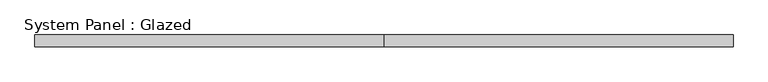
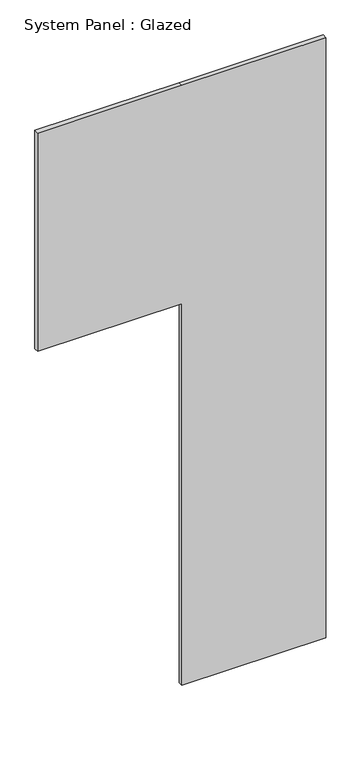
"""IFC4 building model written with IfcOpenShell, lengths in millimetres: plate geometry, System Panel : Glazed."""

from ifc_helpers import new_model, si_unit, frame, origin, place, context, project, spatial, polyline, outline, extrude, source, transform, mapped, element, save


def system_panel_glazed_f04876f4(model_context):
    return source(origin(), model_context, "Body", "SweptSolid", [
        extrude(outline(polyline([(0.0, 0.0), (0.0, 762.0), (2133.6, 762.0), (3352.8, 762.0), (3352.8, 0.0), (3352.8, -762.0), (2133.6, -762.0), (2133.6, 0.0), (0.0, 0.0)])), frame((0.0, 19.05, 0.0), z_axis=(0.0, 1.0, 0.0), x_axis=(0.0, 0.0, 1.0)), (0.0, 0.0, 1.0), 25.4),
    ])


if __name__ == "__main__":
    model = new_model("IFC4")
    model_context = context("Model", 3, world=origin())
    ifc_project = project(units=[si_unit("LENGTHUNIT", "METRE", prefix="MILLI")], contexts=[model_context])
    site = spatial("IfcSite", under=ifc_project)
    building = spatial("IfcBuilding", under=site)
    placement = place(None, origin())
    system_panel_glazed_shape = system_panel_glazed_f04876f4(model_context)
    element("IfcPlate", 1, ObjectType="System Panel : Glazed", at=placement, inside=building, context=model_context, shape_type="MappedRepresentation", body=[
        mapped(system_panel_glazed_shape, transform((0.0, 0.0, 0.0), x_axis=(1.0, 0.0, 0.0), y_axis=(0.0, 1.0, 0.0), z_axis=(0.0, 0.0, 1.0))),
    ])
    save(model, "model.ifc")

# Revit data of these elements
# Type "System Panel : Glazed"
#   Construction Type Id = "GSP4R"
#   Analytic Construction = "1/8 in Pilkington single glazing"
#   Visual Light Transmittance = 0.9
#   Solar Heat Gain Coefficient = 0.86
#   Heat Transfer Coefficient (U) = 1.18115 BTU/(h·ft²·°F)
#   Define Thermal Properties by = 1
# Element 1 (IfcPlate, "System Panel : Glazed")
#   Materials on its faces: "Glass"
# Materials
#   "Glass": class "Glass", colour RGB 0 128 192, transparency 0.75, Description = "Soda Lime Glass", Cost = 0
